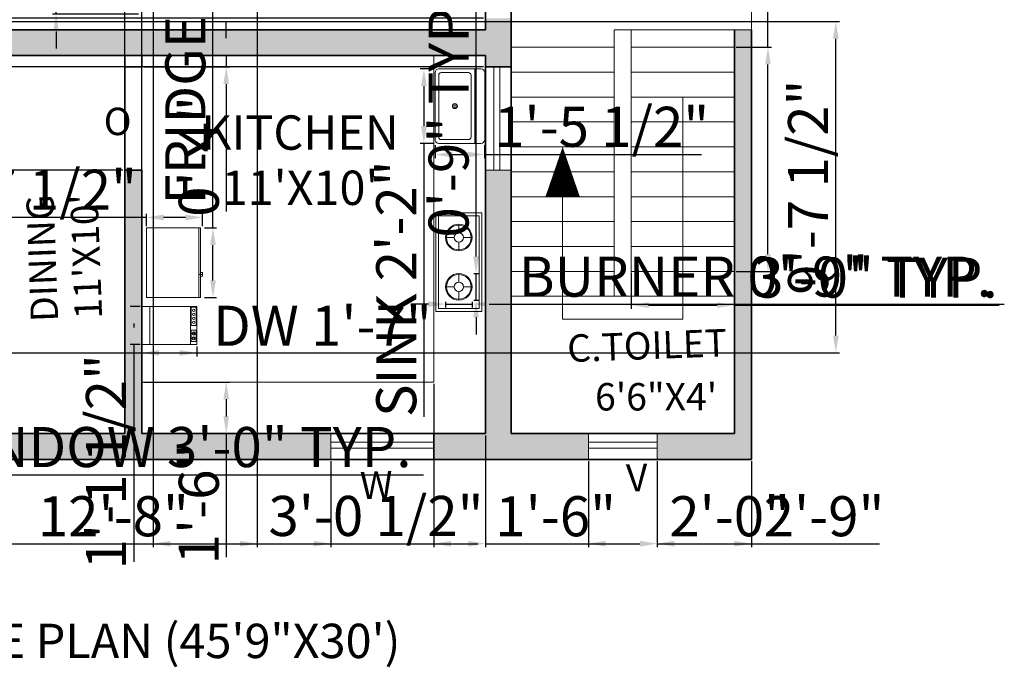
# Model space of a CAD drawing. Units: inches. Extents: x 2961 to 3748, y 1432 to 1961.
# Tile 8 of 9: x 3348 to 3692, y 1432 to 1658. Entities that reach past the tile are written whole.
import ezdxf
from ezdxf.enums import TextEntityAlignment as Align

# ---------------------------------------------------------------- set-up
doc = ezdxf.new("R2010")
doc.units = ezdxf.units.IN
doc.linetypes.add('ACAD_ISO03W100', pattern=[30, 12, -18])
for name, color, linetype, lineweight in [('A-ANNO-DIMS', 2, 'Continuous', 18), ('A-ANNO-TEXT', 7, 'Continuous', 18), ('A-ANNO-TITL', 7, 'Continuous', 25), ('A-AREA-IDEN', 7, 'Continuous', 18), ('A-EQPM', 8, 'Continuous', 18), ('A-FLOR-FIXT', 9, 'Continuous', 18), ('A-FLOR-STRS', 7, 'Continuous', 18), ('A-FURN-FIXD', 9, 'Continuous', 20), ('A-GLAZ', 4, 'Continuous', 18), ('A-ROOF-OVHD', 8, 'ACAD_ISO03W100', 18), ('A-WALL', 7, 'Continuous', 35), ('A-WALL-PATT', 252, 'Continuous', 13)]:
    doc.layers.add(name, color=color, linetype=linetype, lineweight=lineweight)
doc.styles.get("Standard").update_dxf_attribs({"font": 'arial.ttf'})
doc.dimstyles.new('ISO-25', dxfattribs={"dimtxt": 14, "dimasz": 6, "dimexe": 1.25, "dimexo": 0.625, "dimtad": 1, "dimlunit": 3, "dimtxsty": 'Standard', "dimcen": 2.5, "dimadec": 0, "dimazin": 0, "dimtfac": 1, "dimtmove": 0, "dimatfit": 3, "dimfxl": 1, "dimarcsym": 0})

# ---------------------------------------------------------------- blocks, each defined once
blk = doc.blocks.new('Dishwasher')
for p, q in [((16, 32.5), (16.75, 32.5)), ((16.5, 32), (16.2942, 31.7942)), ((16.3156, 33.1843), (16.5, 33)), ((17, 32.75), (17, 33.5)), ((17, 32.25), (17, 31.5)), ((18, 32.5), (17.25, 32.5)), ((17.5, 33), (17.6938, 33.1938)), ((17.7061, 31.7939), (17.5, 32)), ((19, 32.5), (19.75, 32.5)), ((19.5, 32), (19.2942, 31.7942)), ((19.3156, 33.1843), (19.5, 33)), ((20, 32.75), (20, 33.5)), ((20, 32.25), (20, 31.5)), ((21, 32.5), (20.25, 32.5)), ((20.5, 33), (20.6938, 33.1938)), ((20.7061, 31.7939), (20.5, 32)), ((24, 30.5), (0, 30.5)), ((0, 5), (24, 5))]:
    blk.add_line(p, q)
for points in [[(0, 0), (0, 34.5), (24, 34.5), (24, 0)], [(0.5, 31), (0.5, 34), (12, 34), (12, 31)], [(15, 31), (15, 34), (22, 34), (22, 31)]]:
    blk.add_lwpolyline(points, close=True)
for centre, radius in [((2.5, 32.5), 0.75), ((5, 32.5), 0.75), ((7.5, 32.5), 0.75), ((10, 32.5), 0.75), ((17, 32.5), 1), ((20, 32.5), 1)]:
    blk.add_circle(centre, radius)
blk = doc.blocks.new('Refrigerator-2 door - 36 in top')
for p, q in [((0, -26.999999), (36, -26.999999)), ((11, -27.999999), (11, -28.999999)), ((11, -28.999999), (13, -28.999999)), ((12, -26.999999), (12, -28.999999)), ((13, -28.999999), (13, -27.999999))]:
    blk.add_line(p, q)
blk.add_lwpolyline([(0, -27.999999), (0, 0), (36, 0), (36, -27.999999)], close=True)
blk = doc.blocks.new('Sink-single - 30 in top')
blk.add_line((-15, -3.999996), (15, -3.999996))
for points in [[(-13.5, 0), (13.5, 0)], [(-15, -18.499996), (-15, -1.5)], [(15, -1.5), (15, -18.499996)], [(-13.5, -17.499996), (-13.5, -6.499996)], [(-12.5, -5.499996), (12.5, -5.499996)], [(13.5, -6.499996), (13.5, -17.499996)], [(12.5, -18.499996), (-12.5, -18.499996)], [(13.5, -19.999996), (-13.5, -19.999996)]]:
    blk.add_lwpolyline(points)
for radius in [1, 0.5]:
    blk.add_circle((0, -11.999996), radius)
for centre, radius, start, end in [((-13.5, -1.5), 1.5, 90, 180), ((13.5, -1.5), 1.5, 0, 90), ((-12.5, -6.499996), 1, 90, 180), ((12.5, -6.499996), 1, 0, 90), ((-13.5, -18.499996), 1.5, 180, 270), ((-12.5, -17.499996), 1, 180, 270), ((12.5, -17.499996), 1, 270, 0), ((13.5, -18.499996), 1.5, 270, 0)]:
    blk.add_arc(centre, radius, start, end)
blk = doc.blocks.new('WIN-36IN')
for p, q in [((0, 6), (36, 6)), ((0, 3.9), (36, 3.9))]:
    blk.add_line(p, q)
blk.add_lwpolyline([(36, 9), (0, 9), (0, 0), (36, 0)], close=True)
blk = doc.blocks.new('HOB-BURNER')
for p, q in [((4.62, 6.22), (4.62, 9.24)), ((3.02, 4.62), (0, 4.62)), ((9.24, 4.62), (6.22, 4.62)), ((4.62, 0), (4.62, 3.02))]:
    blk.add_line(p, q)
for radius in [4.62, 4.32, 1.6]:
    blk.add_circle((4.62, 4.62), radius)
blk = doc.blocks.new('STAIR-FLIGHT-36IN')
for p, q in [((36, 78.3), (0, 78.3)), ((36, 69.6), (0, 69.6)), ((36, 60.9), (0, 60.9)), ((36, 52.2), (0, 52.2)), ((36, 43.5), (0, 43.5)), ((36, 34.8), (0, 34.8)), ((36, 26.1), (0, 26.1)), ((36, 17.4), (0, 17.4)), ((36, 8.7), (0, 8.7)), ((36, 0), (0, 0)), ((36, 0), (0, 0))]:
    blk.add_line(p, q)
blk = doc.blocks.new('*D20')
at = {"layer": 'A-ANNO-DIMS', "color": 0, "lineweight": -2, "transparency": 16777216}
for p, q in [((3268.27, 1504.01), (3268.27, 1497.99)), ((3304.27, 1504.01), (3304.27, 1497.99)), ((3274.27, 1499.24), (3298.27, 1499.24)), ((3304.27, 1499.24), (3488.68, 1499.24))]:
    blk.add_line(p, q, dxfattribs=at)
at = {"layer": 'A-ANNO-DIMS', "color": 0, "transparency": 16777216}
for points in [[(3274.27, 1500.24), (3274.27, 1498.24), (3268.27, 1499.24)], [(3298.27, 1500.24), (3298.27, 1498.24), (3304.27, 1499.24)]]:
    blk.add_solid(points, dxfattribs=at)
at = {"layer": 'Defpoints', "color": 0, "transparency": 16777216}
for p in [(3268.27, 1504.64), (3304.27, 1504.64), (3304.27, 1499.24)]:
    blk.add_point(p, dxfattribs=at)
at = {"layer": 'A-ANNO-DIMS', "color": 0, "transparency": 16777216, "insert": (3399.47, 1507.11), "char_height": 14, "attachment_point": 5}
blk.add_mtext('WINDOW 3\'-0" TYP.', dxfattribs=at)
blk = doc.blocks.new('*D34')
at = {"layer": 'A-ANNO-DIMS', "color": 0, "lineweight": -2, "transparency": 16777216}
for p, q in [((3490.37, 1558.86), (3484.37, 1558.86)), ((3496.37, 1559.62), (3496.37, 1557.61)), ((3496.37, 1558.86), (3505.61, 1558.86)), ((3505.61, 1559.62), (3505.61, 1557.61)), ((3511.61, 1558.86), (3691.6, 1558.86))]:
    blk.add_line(p, q, dxfattribs=at)
at = {"layer": 'A-ANNO-DIMS', "color": 0, "transparency": 16777216}
for points in [[(3490.37, 1559.86), (3490.37, 1557.86), (3496.37, 1558.86)], [(3511.61, 1559.86), (3511.61, 1557.86), (3505.61, 1558.86)]]:
    blk.add_solid(points, dxfattribs=at)
at = {"layer": 'Defpoints', "color": 0, "transparency": 16777216}
for p in [(3496.37, 1560.25), (3505.61, 1560.25), (3505.61, 1558.86)]:
    blk.add_point(p, dxfattribs=at)
at = {"layer": 'A-ANNO-DIMS', "color": 0, "transparency": 16777216, "insert": (3604.6, 1566.63), "char_height": 14, "attachment_point": 5}
blk.add_mtext('BURNER 0\'-9" TYP.', dxfattribs=at)
blk = doc.blocks.new('*D35')
at = {"layer": 'A-ANNO-DIMS', "color": 0, "lineweight": -2, "transparency": 16777216}
for p, q in [((3507, 1575.49), (3507, 1668.08)), ((3506.23, 1569.49), (3508.25, 1569.49)), ((3507, 1560.25), (3507, 1569.49)), ((3506.23, 1560.25), (3508.25, 1560.25)), ((3507, 1554.25), (3507, 1548.25))]:
    blk.add_line(p, q, dxfattribs=at)
at = {"layer": 'A-ANNO-DIMS', "color": 0, "transparency": 16777216}
for points in [[(3506, 1575.49), (3508, 1575.49), (3507, 1569.49)], [(3506, 1554.25), (3508, 1554.25), (3507, 1560.25)]]:
    blk.add_solid(points, dxfattribs=at)
at = {"layer": 'Defpoints', "color": 0, "transparency": 16777216}
for p in [(3505.61, 1569.49), (3507, 1569.49), (3505.61, 1560.25)]:
    blk.add_point(p, dxfattribs=at)
at = {"layer": 'A-ANNO-DIMS', "color": 0, "transparency": 16777216, "insert": (3499.22, 1624.78), "char_height": 14, "attachment_point": 5, "rotation": 90}
blk.add_mtext('0\'-9" TYP.', dxfattribs=at)
blk = doc.blocks.new('*D36')
at = {"layer": 'A-ANNO-DIMS', "color": 0, "lineweight": -2, "transparency": 16777216}
for p, q in [((3609.01, 1648.54), (3609.01, 1911.68)), ((3597.89, 1648.54), (3610.26, 1648.54)), ((3609.01, 1576.24), (3609.01, 1642.54)), ((3597.89, 1570.24), (3610.26, 1570.24))]:
    blk.add_line(p, q, dxfattribs=at)
at = {"layer": 'A-ANNO-DIMS', "color": 0, "transparency": 16777216}
for points in [[(3608.01, 1642.54), (3610.01, 1642.54), (3609.01, 1648.54)], [(3608.01, 1576.24), (3610.01, 1576.24), (3609.01, 1570.24)]]:
    blk.add_solid(points, dxfattribs=at)
at = {"layer": 'Defpoints', "color": 0, "transparency": 16777216}
for p in [(3597.27, 1648.54), (3609.01, 1648.54), (3597.27, 1570.24)]:
    blk.add_point(p, dxfattribs=at)
at = {"layer": 'A-ANNO-DIMS', "color": 0, "transparency": 16777216, "insert": (3601.15, 1783.11), "char_height": 14, "attachment_point": 5, "rotation": 90}
blk.add_mtext('STAIR FLIGHT 6\'-6 1/2" TYP.', dxfattribs=at)
blk = doc.blocks.new('*D37')
at = {"layer": 'A-ANNO-DIMS', "color": 0, "lineweight": -2, "transparency": 16777216}
for p, q in [((3561.27, 1569.61), (3561.27, 1557.24)), ((3597.27, 1569.61), (3597.27, 1557.24)), ((3567.27, 1558.49), (3591.27, 1558.49)), ((3597.27, 1558.49), (3689.84, 1558.49))]:
    blk.add_line(p, q, dxfattribs=at)
at = {"layer": 'A-ANNO-DIMS', "color": 0, "transparency": 16777216}
for points in [[(3567.27, 1559.49), (3567.27, 1557.49), (3561.27, 1558.49)], [(3591.27, 1559.49), (3591.27, 1557.49), (3597.27, 1558.49)]]:
    blk.add_solid(points, dxfattribs=at)
at = {"layer": 'Defpoints', "color": 0, "transparency": 16777216}
for p in [(3561.27, 1570.24), (3597.27, 1570.24), (3597.27, 1558.49)]:
    blk.add_point(p, dxfattribs=at)
at = {"layer": 'A-ANNO-DIMS', "color": 0, "transparency": 16777216, "insert": (3646.56, 1566.27), "char_height": 14, "attachment_point": 5}
blk.add_mtext('3\'-0" TYP.', dxfattribs=at)
blk = doc.blocks.new('*D38')
at = {"layer": 'A-ANNO-DIMS', "color": 0, "lineweight": -2, "transparency": 16777216}
for p, q in [((3390.27, 1544.05), (3390.27, 1540.55)), ((3396.27, 1541.8), (3403.45, 1541.8)), ((3409.45, 1544.05), (3409.45, 1540.55)), ((3409.45, 1541.8), (3491.24, 1541.8))]:
    blk.add_line(p, q, dxfattribs=at)
at = {"layer": 'A-ANNO-DIMS', "color": 0, "transparency": 16777216}
for points in [[(3396.27, 1542.8), (3396.27, 1540.8), (3390.27, 1541.8)], [(3403.45, 1542.8), (3403.45, 1540.8), (3409.45, 1541.8)]]:
    blk.add_solid(points, dxfattribs=at)
at = {"layer": 'Defpoints', "color": 0, "transparency": 16777216}
for p in [(3390.27, 1544.68), (3409.45, 1544.68), (3409.45, 1541.8)]:
    blk.add_point(p, dxfattribs=at)
at = {"layer": 'A-ANNO-DIMS', "color": 0, "transparency": 16777216, "insert": (3453.35, 1549.46), "char_height": 14, "attachment_point": 5}
blk.add_mtext('DW 1\'-7"', dxfattribs=at)
blk = doc.blocks.new('*D39')
at = {"layer": 'A-ANNO-DIMS', "color": 0, "lineweight": -2, "transparency": 16777216}
for p, q in [((3389.64, 1558.03), (3386.14, 1558.03)), ((3387.39, 1552.03), (3387.39, 1550.68)), ((3389.64, 1544.68), (3386.14, 1544.68)), ((3387.39, 1544.68), (3387.39, 1468.91))]:
    blk.add_line(p, q, dxfattribs=at)
at = {"layer": 'A-ANNO-DIMS', "color": 0, "transparency": 16777216}
for points in [[(3386.39, 1552.03), (3388.39, 1552.03), (3387.39, 1558.03)], [(3386.39, 1550.68), (3388.39, 1550.68), (3387.39, 1544.68)]]:
    blk.add_solid(points, dxfattribs=at)
at = {"layer": 'Defpoints', "color": 0, "transparency": 16777216}
for p in [(3390.27, 1558.03), (3387.39, 1544.68), (3390.27, 1544.68)]:
    blk.add_point(p, dxfattribs=at)
at = {"layer": 'A-ANNO-DIMS', "color": 0, "transparency": 16777216, "insert": (3379.52, 1503.79), "char_height": 14, "attachment_point": 5, "rotation": 90}
blk.add_mtext('1\'-1 1/2"', dxfattribs=at)
blk = doc.blocks.new('*D40')
at = {"layer": 'A-ANNO-DIMS', "color": 0, "lineweight": -2, "transparency": 16777216}
for p, q in [((3415.09, 1585.45), (3415.09, 1741.07)), ((3412.07, 1585.45), (3416.34, 1585.45)), ((3415.09, 1567.11), (3415.09, 1579.45)), ((3412.07, 1561.11), (3416.34, 1561.11))]:
    blk.add_line(p, q, dxfattribs=at)
at = {"layer": 'A-ANNO-DIMS', "color": 0, "transparency": 16777216}
for points in [[(3414.09, 1579.45), (3416.09, 1579.45), (3415.09, 1585.45)], [(3414.09, 1567.11), (3416.09, 1567.11), (3415.09, 1561.11)]]:
    blk.add_solid(points, dxfattribs=at)
at = {"layer": 'Defpoints', "color": 0, "transparency": 16777216}
for p in [(3411.44, 1585.45), (3415.09, 1585.45), (3411.44, 1561.11)]:
    blk.add_point(p, dxfattribs=at)
at = {"layer": 'A-ANNO-DIMS', "color": 0, "transparency": 16777216, "insert": (3407.23, 1666.26), "char_height": 14, "attachment_point": 5, "rotation": 90}
blk.add_mtext('FRIDGE 2\'-0 1/2"', dxfattribs=at)
blk = doc.blocks.new('*D41')
at = {"layer": 'A-ANNO-DIMS', "color": 0, "lineweight": -2, "transparency": 16777216}
for p, q in [((3391.84, 1586.08), (3391.84, 1590.35)), ((3411.44, 1586.08), (3411.44, 1590.35)), ((3391.84, 1589.1), (3316.07, 1589.1)), ((3405.44, 1589.1), (3397.84, 1589.1))]:
    blk.add_line(p, q, dxfattribs=at)
at = {"layer": 'A-ANNO-DIMS', "color": 0, "transparency": 16777216}
for points in [[(3397.84, 1590.1), (3397.84, 1588.1), (3391.84, 1589.1)], [(3405.44, 1590.1), (3405.44, 1588.1), (3411.44, 1589.1)]]:
    blk.add_solid(points, dxfattribs=at)
at = {"layer": 'Defpoints', "color": 0, "transparency": 16777216}
for p in [(3391.84, 1589.1), (3391.84, 1585.45), (3411.44, 1585.45)]:
    blk.add_point(p, dxfattribs=at)
at = {"layer": 'A-ANNO-DIMS', "color": 0, "transparency": 16777216, "insert": (3350.95, 1596.96), "char_height": 14, "attachment_point": 5}
blk.add_mtext('1\'-7 1/2"', dxfattribs=at)
blk = doc.blocks.new('*D42')
at = {"layer": 'A-ANNO-DIMS', "color": 0, "lineweight": -2, "transparency": 16777216}
for p, q in [((3492.07, 1640.96), (3487.54, 1640.96)), ((3488.79, 1634.96), (3488.79, 1620.96)), ((3492.07, 1614.96), (3487.54, 1614.96)), ((3488.79, 1614.96), (3488.79, 1519.48))]:
    blk.add_line(p, q, dxfattribs=at)
at = {"layer": 'A-ANNO-DIMS', "color": 0, "transparency": 16777216}
for points in [[(3487.79, 1634.96), (3489.79, 1634.96), (3488.79, 1640.96)], [(3487.79, 1620.96), (3489.79, 1620.96), (3488.79, 1614.96)]]:
    blk.add_solid(points, dxfattribs=at)
at = {"layer": 'Defpoints', "color": 0, "transparency": 16777216}
for p in [(3492.69, 1640.96), (3488.79, 1614.96), (3492.69, 1614.96)]:
    blk.add_point(p, dxfattribs=at)
at = {"layer": 'A-ANNO-DIMS', "color": 0, "transparency": 16777216, "insert": (3480.93, 1564.22), "char_height": 14, "attachment_point": 5, "rotation": 90}
blk.add_mtext('SINK 2\'-2"', dxfattribs=at)
blk = doc.blocks.new('*D43')
at = {"layer": 'A-ANNO-DIMS', "color": 0, "lineweight": -2, "transparency": 16777216}
for p, q in [((3492.69, 1614.34), (3492.69, 1609.81)), ((3510.02, 1614.34), (3510.02, 1609.81)), ((3498.69, 1611.06), (3504.02, 1611.06)), ((3510.02, 1611.06), (3585.79, 1611.06))]:
    blk.add_line(p, q, dxfattribs=at)
at = {"layer": 'A-ANNO-DIMS', "color": 0, "transparency": 16777216}
for points in [[(3498.69, 1612.06), (3498.69, 1610.06), (3492.69, 1611.06)], [(3504.02, 1612.06), (3504.02, 1610.06), (3510.02, 1611.06)]]:
    blk.add_solid(points, dxfattribs=at)
at = {"layer": 'Defpoints', "color": 0, "transparency": 16777216}
for p in [(3492.69, 1614.96), (3510.02, 1614.96), (3510.02, 1611.06)]:
    blk.add_point(p, dxfattribs=at)
at = {"layer": 'A-ANNO-DIMS', "color": 0, "transparency": 16777216, "insert": (3550.91, 1618.93), "char_height": 14, "attachment_point": 5}
blk.add_mtext('1\'-5 1/2"', dxfattribs=at)
blk = doc.blocks.new('*D51')
at = {"layer": 'A-ANNO-DIMS', "color": 0, "lineweight": -2, "transparency": 16777216}
for p, q in [((3390.89, 1531.64), (3420.97, 1531.64)), ((3419.72, 1525.64), (3419.72, 1519.64)), ((3390.89, 1513.64), (3420.97, 1513.64)), ((3419.72, 1513.64), (3419.72, 1470.49))]:
    blk.add_line(p, q, dxfattribs=at)
at = {"layer": 'A-ANNO-DIMS', "color": 0, "transparency": 16777216}
for points in [[(3418.72, 1525.64), (3420.72, 1525.64), (3419.72, 1531.64)], [(3418.72, 1519.64), (3420.72, 1519.64), (3419.72, 1513.64)]]:
    blk.add_solid(points, dxfattribs=at)
at = {"layer": 'Defpoints', "color": 0, "transparency": 16777216}
for p in [(3390.27, 1531.64), (3390.27, 1513.64), (3419.72, 1513.64)]:
    blk.add_point(p, dxfattribs=at)
at = {"layer": 'A-ANNO-DIMS', "color": 0, "transparency": 16777216, "insert": (3411.94, 1489.06), "char_height": 14, "attachment_point": 5, "rotation": 90}
blk.add_mtext('1\'-6"', dxfattribs=at)
blk = doc.blocks.new('*D52')
at = {"layer": 'A-ANNO-DIMS', "color": 0, "lineweight": -2, "transparency": 16777216}
for p, q in [((3360.27, 1678.21), (3360.27, 1721.36)), ((3389.1, 1672.21), (3359.02, 1672.21)), ((3360.27, 1660.05), (3360.27, 1672.21)), ((3389.1, 1660.05), (3359.02, 1660.05)), ((3360.27, 1654.05), (3360.27, 1648.05))]:
    blk.add_line(p, q, dxfattribs=at)
at = {"layer": 'A-ANNO-DIMS', "color": 0, "transparency": 16777216}
for points in [[(3359.27, 1678.21), (3361.27, 1678.21), (3360.27, 1672.21)], [(3359.27, 1654.05), (3361.27, 1654.05), (3360.27, 1660.05)]]:
    blk.add_solid(points, dxfattribs=at)
at = {"layer": 'Defpoints', "color": 0, "transparency": 16777216}
for p in [(3360.27, 1672.21), (3389.72, 1672.21), (3389.72, 1660.05)]:
    blk.add_point(p, dxfattribs=at)
at = {"layer": 'A-ANNO-DIMS', "color": 0, "transparency": 16777216, "insert": (3352.5, 1702.78), "char_height": 14, "attachment_point": 5, "rotation": 90}
blk.add_mtext('1\'-0"', dxfattribs=at)
blk = doc.blocks.new('*D58')
at = {"layer": 'A-ANNO-DIMS', "color": 0, "lineweight": -2, "transparency": 16777216}
for p, q in [((3304.27, 1504.01), (3304.27, 1473.94)), ((3456.27, 1504.01), (3456.27, 1473.94)), ((3310.27, 1475.19), (3450.27, 1475.19))]:
    blk.add_line(p, q, dxfattribs=at)
at = {"layer": 'A-ANNO-DIMS', "color": 0, "transparency": 16777216}
for points in [[(3310.27, 1476.19), (3310.27, 1474.19), (3304.27, 1475.19)], [(3450.27, 1476.19), (3450.27, 1474.19), (3456.27, 1475.19)]]:
    blk.add_solid(points, dxfattribs=at)
at = {"layer": 'Defpoints', "color": 0, "transparency": 16777216}
for p in [(3304.27, 1504.64), (3456.27, 1504.64), (3456.27, 1475.19)]:
    blk.add_point(p, dxfattribs=at)
at = {"layer": 'A-ANNO-DIMS', "color": 0, "transparency": 16777216, "insert": (3380.27, 1482.96), "char_height": 14, "attachment_point": 5}
blk.add_mtext('12\'-8"', dxfattribs=at)
blk = doc.blocks.new('*D59')
at = {"layer": 'A-ANNO-DIMS', "color": 0, "lineweight": -2, "transparency": 16777216}
for p, q in [((3570.27, 1504.01), (3570.27, 1473.94)), ((3603.27, 1504.01), (3603.27, 1473.94)), ((3576.27, 1475.19), (3597.27, 1475.19)), ((3603.27, 1475.19), (3647.97, 1475.19))]:
    blk.add_line(p, q, dxfattribs=at)
at = {"layer": 'A-ANNO-DIMS', "color": 0, "transparency": 16777216}
for points in [[(3576.27, 1476.19), (3576.27, 1474.19), (3570.27, 1475.19)], [(3597.27, 1476.19), (3597.27, 1474.19), (3603.27, 1475.19)]]:
    blk.add_solid(points, dxfattribs=at)
at = {"layer": 'Defpoints', "color": 0, "transparency": 16777216}
for p in [(3570.27, 1504.64), (3603.27, 1504.64), (3603.27, 1475.19)]:
    blk.add_point(p, dxfattribs=at)
at = {"layer": 'A-ANNO-DIMS', "color": 0, "transparency": 16777216, "insert": (3628.62, 1482.96), "char_height": 14, "attachment_point": 5}
blk.add_mtext('2\'-9"', dxfattribs=at)
blk = doc.blocks.new('*D60')
at = {"layer": 'A-ANNO-DIMS', "color": 0, "lineweight": -2, "transparency": 16777216}
for p, q in [((3546.27, 1504.01), (3546.27, 1473.94)), ((3570.27, 1504.01), (3570.27, 1473.94)), ((3552.27, 1475.19), (3564.27, 1475.19)), ((3570.27, 1475.19), (3614.97, 1475.19))]:
    blk.add_line(p, q, dxfattribs=at)
at = {"layer": 'A-ANNO-DIMS', "color": 0, "transparency": 16777216}
for points in [[(3552.27, 1476.19), (3552.27, 1474.19), (3546.27, 1475.19)], [(3564.27, 1476.19), (3564.27, 1474.19), (3570.27, 1475.19)]]:
    blk.add_solid(points, dxfattribs=at)
at = {"layer": 'Defpoints', "color": 0, "transparency": 16777216}
for p in [(3546.27, 1504.64), (3570.27, 1504.64), (3570.27, 1475.19)]:
    blk.add_point(p, dxfattribs=at)
at = {"layer": 'A-ANNO-DIMS', "color": 0, "transparency": 16777216, "insert": (3595.62, 1482.96), "char_height": 14, "attachment_point": 5}
blk.add_mtext('2\'-0"', dxfattribs=at)
blk = doc.blocks.new('*D68')
at = {"layer": 'A-ANNO-DIMS', "color": 0, "lineweight": -2, "transparency": 16777216}
for p, q in [((3024.82, 1658.64), (3024.82, 1701.79)), ((3509.64, 1658.64), (3023.57, 1658.64)), ((3024.82, 1647.64), (3024.82, 1652.64)), ((3509.64, 1641.64), (3023.57, 1641.64))]:
    blk.add_line(p, q, dxfattribs=at)
at = {"layer": 'A-ANNO-DIMS', "color": 0, "transparency": 16777216}
for points in [[(3023.82, 1652.64), (3025.82, 1652.64), (3024.82, 1658.64)], [(3023.82, 1647.64), (3025.82, 1647.64), (3024.82, 1641.64)]]:
    blk.add_solid(points, dxfattribs=at)
at = {"layer": 'Defpoints', "color": 0, "transparency": 16777216}
for p in [(3024.82, 1658.64), (3510.27, 1658.64), (3510.27, 1641.64)]:
    blk.add_point(p, dxfattribs=at)
at = {"layer": 'A-ANNO-DIMS', "color": 0, "transparency": 16777216, "insert": (3017.04, 1683.21), "char_height": 14, "attachment_point": 5, "rotation": 90}
blk.add_mtext('1\'-5"', dxfattribs=at)
blk = doc.blocks.new('*D70')
at = {"layer": 'A-ANNO-DIMS', "color": 0, "lineweight": -2, "transparency": 16777216}
for p, q in [((3024.82, 1641.64), (3024.82, 1686.09)), ((3383.64, 1641.64), (3023.57, 1641.64)), ((3024.82, 1611.64), (3024.82, 1635.64)), ((3383.64, 1605.64), (3023.57, 1605.64))]:
    blk.add_line(p, q, dxfattribs=at)
at = {"layer": 'A-ANNO-DIMS', "color": 0, "transparency": 16777216}
for points in [[(3023.82, 1635.64), (3025.82, 1635.64), (3024.82, 1641.64)], [(3023.82, 1611.64), (3025.82, 1611.64), (3024.82, 1605.64)]]:
    blk.add_solid(points, dxfattribs=at)
at = {"layer": 'Defpoints', "color": 0, "transparency": 16777216}
for p in [(3024.82, 1641.64), (3384.27, 1641.64), (3384.27, 1605.64)]:
    blk.add_point(p, dxfattribs=at)
at = {"layer": 'A-ANNO-DIMS', "color": 0, "transparency": 16777216, "insert": (3017.04, 1666.87), "char_height": 14, "attachment_point": 5, "rotation": 90}
blk.add_mtext('3\'-0"', dxfattribs=at)
blk = doc.blocks.new('*D78')
at = {"layer": 'A-ANNO-DIMS', "color": 0, "lineweight": -2, "transparency": 16777216}
for p, q in [((3394.23, 1792.44), (3394.23, 1473.94)), ((3430.5, 1792.44), (3430.5, 1473.94)), ((3400.23, 1475.19), (3424.5, 1475.19)), ((3430.5, 1475.19), (3507.58, 1475.19))]:
    blk.add_line(p, q, dxfattribs=at)
at = {"layer": 'A-ANNO-DIMS', "color": 0, "transparency": 16777216}
for points in [[(3400.23, 1476.19), (3400.23, 1474.19), (3394.23, 1475.19)], [(3424.5, 1476.19), (3424.5, 1474.19), (3430.5, 1475.19)]]:
    blk.add_solid(points, dxfattribs=at)
at = {"layer": 'Defpoints', "color": 0, "transparency": 16777216}
for p in [(3394.23, 1793.06), (3430.5, 1793.06), (3430.5, 1475.19)]:
    blk.add_point(p, dxfattribs=at)
at = {"layer": 'A-ANNO-DIMS', "color": 0, "transparency": 16777216, "insert": (3472.04, 1483.06), "char_height": 14, "attachment_point": 5}
blk.add_mtext('3\'-0 1/2"', dxfattribs=at)
blk = doc.blocks.new('*D81')
at = {"layer": 'A-ANNO-DIMS', "color": 0, "lineweight": -2, "transparency": 16777216}
for p, q in [((3063.89, 1657.48), (3633.97, 1657.48)), ((3632.72, 1547.87), (3632.72, 1651.48)), ((3063.89, 1541.87), (3633.97, 1541.87))]:
    blk.add_line(p, q, dxfattribs=at)
at = {"layer": 'A-ANNO-DIMS', "color": 0, "transparency": 16777216}
for points in [[(3631.72, 1651.48), (3633.72, 1651.48), (3632.72, 1657.48)], [(3631.72, 1547.87), (3633.72, 1547.87), (3632.72, 1541.87)]]:
    blk.add_solid(points, dxfattribs=at)
at = {"layer": 'Defpoints', "color": 0, "transparency": 16777216}
for p in [(3063.27, 1657.48), (3632.72, 1657.48), (3063.27, 1541.87)]:
    blk.add_point(p, dxfattribs=at)
at = {"layer": 'A-ANNO-DIMS', "color": 0, "transparency": 16777216, "insert": (3624.85, 1599.67), "char_height": 14, "attachment_point": 5, "rotation": 90}
blk.add_mtext('9\'-7 1/2"', dxfattribs=at)
blk = doc.blocks.new('*D87')
at = {"layer": 'A-ANNO-DIMS', "color": 0, "lineweight": -2, "transparency": 16777216}
for p, q in [((3384.27, 1514.26), (3384.27, 1933.63)), ((3390.27, 1514.26), (3390.27, 1933.63)), ((3378.27, 1932.38), (3372.27, 1932.38)), ((3384.27, 1932.38), (3390.27, 1932.38)), ((3396.27, 1932.38), (3440.73, 1932.38))]:
    blk.add_line(p, q, dxfattribs=at)
at = {"layer": 'A-ANNO-DIMS', "color": 0, "transparency": 16777216}
for points in [[(3378.27, 1933.38), (3378.27, 1931.38), (3384.27, 1932.38)], [(3396.27, 1933.38), (3396.27, 1931.38), (3390.27, 1932.38)]]:
    blk.add_solid(points, dxfattribs=at)
at = {"layer": 'Defpoints', "color": 0, "transparency": 16777216}
for p in [(3390.27, 1932.38), (3384.27, 1513.64), (3390.27, 1513.64)]:
    blk.add_point(p, dxfattribs=at)
at = {"layer": 'A-ANNO-DIMS', "color": 0, "transparency": 16777216, "insert": (3421.5, 1940.15), "char_height": 14, "attachment_point": 5}
blk.add_mtext('0\'-6"', dxfattribs=at)
blk = doc.blocks.new('*D88')
at = {"layer": 'A-ANNO-DIMS', "color": 0, "lineweight": -2, "transparency": 16777216}
for p, q in [((3492.27, 1531.01), (3492.27, 1473.94)), ((3510.27, 1513.01), (3510.27, 1473.94)), ((3498.27, 1475.19), (3504.27, 1475.19)), ((3510.27, 1475.19), (3553.41, 1475.19))]:
    blk.add_line(p, q, dxfattribs=at)
at = {"layer": 'A-ANNO-DIMS', "color": 0, "transparency": 16777216}
for points in [[(3498.27, 1476.19), (3498.27, 1474.19), (3492.27, 1475.19)], [(3504.27, 1476.19), (3504.27, 1474.19), (3510.27, 1475.19)]]:
    blk.add_solid(points, dxfattribs=at)
at = {"layer": 'Defpoints', "color": 0, "transparency": 16777216}
for p in [(3492.27, 1531.64), (3510.27, 1513.64), (3510.27, 1475.19)]:
    blk.add_point(p, dxfattribs=at)
at = {"layer": 'A-ANNO-DIMS', "color": 0, "transparency": 16777216, "insert": (3534.84, 1482.96), "char_height": 14, "attachment_point": 5}
blk.add_mtext('1\'-6"', dxfattribs=at)
blk = doc.blocks.new('*D90')
at = {"layer": 'A-ANNO-DIMS', "color": 0, "lineweight": -2, "transparency": 16777216}
for p, q in [((3419.72, 1651.64), (3419.72, 1657.64)), ((3390.89, 1645.64), (3420.97, 1645.64)), ((3419.72, 1645.64), (3419.72, 1641.64)), ((3390.89, 1641.64), (3420.97, 1641.64)), ((3419.72, 1635.64), (3419.72, 1591.17))]:
    blk.add_line(p, q, dxfattribs=at)
at = {"layer": 'A-ANNO-DIMS', "color": 0, "transparency": 16777216}
for points in [[(3418.72, 1651.64), (3420.72, 1651.64), (3419.72, 1645.64)], [(3418.72, 1635.64), (3420.72, 1635.64), (3419.72, 1641.64)]]:
    blk.add_solid(points, dxfattribs=at)
at = {"layer": 'Defpoints', "color": 0, "transparency": 16777216}
for p in [(3390.27, 1645.64), (3390.27, 1641.64), (3419.72, 1641.64)]:
    blk.add_point(p, dxfattribs=at)
at = {"layer": 'A-ANNO-DIMS', "color": 0, "transparency": 16777216, "insert": (3411.94, 1610.41), "char_height": 14, "attachment_point": 5, "rotation": 90}
blk.add_mtext('0\'-4"', dxfattribs=at)

msp = doc.modelspace()

# ---------------------------------------------------------------- hatches: boundary and pattern name
at = {"layer": 'A-WALL-PATT'}
h = msp.add_hatch(color=256, dxfattribs=at)
h.set_gradient(color1=(41, 49, 137), color2=(41, 49, 137), tint=1)
h.paths.add_polyline_path([(3255.267, 1671.639), (3255.267, 1513.639), (3251.267, 1513.639), (3251.267, 1504.639), (3268.267, 1504.639), (3268.267, 1513.639), (3264.267, 1513.639), (3264.267, 1671.639), (3259.767, 1671.639)])
h.paths.add_polyline_path([(3063.267, 1513.639), (3063.267, 1677.639), (3054.267, 1677.639), (3054.267, 1504.639), (3215.267, 1504.639), (3215.267, 1513.639)])
h.paths.add_polyline_path([(3304.267, 1513.639), (3304.267, 1504.639), (3456.267, 1504.639), (3456.267, 1513.639), (3390.267, 1513.639), (3390.267, 1605.639), (3384.267, 1605.639), (3384.267, 1513.639)])
h.paths.add_polyline_path([(3510.267, 1605.639), (3510.267, 1513.639), (3492.267, 1513.639), (3492.267, 1504.639), (3546.267, 1504.639), (3546.267, 1513.639), (3519.267, 1513.639), (3519.267, 1605.639)])
h.paths.add_polyline_path([(3340.267, 1654.639), (3340.267, 1645.639), (3510.267, 1645.639), (3510.267, 1641.639), (3519.267, 1641.639), (3519.267, 1658.639), (3510.267, 1658.639), (3510.267, 1654.639)])
h.paths.add_polyline_path([(3223.801, 1864.639), (3223.801, 1855.639), (3255.267, 1855.639), (3255.267, 1772.534), (3264.267, 1772.534), (3264.267, 1855.639), (3303.267, 1855.639), (3303.267, 1864.639)])
h.paths.add_polyline_path([(3339.267, 1864.639), (3339.267, 1855.639), (3435.267, 1855.639), (3435.267, 1864.639)])
h.paths.add_polyline_path([(3471.267, 1864.639), (3471.267, 1855.639), (3510.267, 1855.639), (3510.267, 1827.639), (3519.267, 1827.639), (3519.267, 1864.639)])
h.paths.add_polyline_path([(3510.267, 1767.639), (3510.267, 1739.639), (3519.267, 1739.639), (3519.267, 1767.639)])
h.paths.add_polyline_path([(3123.267, 1726.639), (3123.267, 1855.639), (3187.801, 1855.639), (3187.801, 1864.639), (3054.267, 1864.639), (3054.267, 1837.201), (3063.267, 1837.201), (3063.267, 1855.639), (3117.267, 1855.639), (3117.267, 1726.639), (3103.267, 1726.639), (3103.267, 1717.639), (3255.267, 1717.639), (3255.267, 1713.639), (3264.267, 1713.639), (3264.267, 1730.534), (3255.267, 1730.639), (3255.267, 1726.639)])
h.paths.add_polyline_path([(3597.267, 1654.639), (3597.267, 1513.639), (3570.267, 1513.639), (3570.267, 1504.639), (3603.267, 1504.639), (3603.267, 1654.639)])
h.paths.add_polyline_path([(3054.267, 1813.201), (3054.267, 1713.639), (3063.267, 1713.639), (3063.267, 1717.639), (3069.267, 1717.639), (3069.267, 1726.639), (3063.267, 1726.639), (3063.267, 1813.201)], flags=17)

# ---------------------------------------------------------------- linework, layer by layer
at = {"layer": 'A-EQPM'}
for points in [[(3492.912, 1556.259), (3492.912, 1590.698), (3509.063, 1590.698), (3509.063, 1556.259)], [(3493.912, 1557.259), (3493.912, 1589.698), (3508.063, 1589.698), (3508.063, 1557.259)]]:
    msp.add_lwpolyline(points, close=True, dxfattribs=at)
at = {"layer": 'A-FLOR-STRS'}
for p, q in [((3603.267, 1654.639), (3555.267, 1654.639)), ((3555.267, 1561.639), (3555.267, 1654.639)), ((3561.267, 1561.639), (3561.267, 1654.639)), ((3579.267, 1631.139), (3579.267, 1561.639)), ((3537.267, 1553.526), (3537.267, 1596.339)), ((3597.267, 1561.639), (3519.267, 1561.639)), ((3579.267, 1561.639), (3579.267, 1553.526)), ((3579.267, 1553.526), (3537.267, 1553.526))]:
    msp.add_line(p, q, dxfattribs=at)
msp.add_lwpolyline([(3537.267, 1596.339, 12, 0, 0), (3537.267, 1613.739, 0, 0, 0)], format="xyseb", dxfattribs=at)
at = {"layer": 'A-FURN-FIXD'}
for p in [(3492.267, 1645.639), (3390.267, 1531.639)]:
    msp.add_line(p, (3492.267, 1531.639), dxfattribs=at)
at = {"layer": 'A-GLAZ'}
for p, q in [((3546.267, 1510.639), (3570.267, 1510.639)), ((3546.267, 1508.539), (3570.267, 1508.539))]:
    msp.add_line(p, q, dxfattribs=at)
msp.add_lwpolyline([(3546.267, 1513.639), (3546.267, 1504.639), (3570.267, 1504.639), (3570.267, 1513.639)], close=True, dxfattribs=at)
at = {"layer": 'A-ROOF-OVHD'}
msp.add_line((3603.267, 1654.639), (3603.267, 1864.639), dxfattribs=at)
at = {"layer": 'A-WALL'}
for p, q in [((3519.267, 1513.639), (3519.267, 1864.639)), ((3510.267, 1654.639), (3510.267, 1767.639)), ((3510.267, 1654.639), (3264.267, 1654.639)), ((3597.267, 1513.639), (3597.267, 1654.639)), ((3603.267, 1504.639), (3603.267, 1654.639)), ((3510.267, 1645.639), (3340.267, 1645.639)), ((3384.267, 1513.639), (3384.267, 1645.639)), ((3390.267, 1641.639), (3390.267, 1645.639)), ((3510.267, 1513.639), (3510.267, 1645.639)), ((3390.267, 1641.639), (3384.267, 1641.639)), ((3510.267, 1641.639), (3519.267, 1641.639)), ((3390.267, 1605.639), (3384.267, 1605.639)), ((3390.267, 1513.639), (3390.267, 1605.639)), ((3384.267, 1513.639), (3264.267, 1513.639)), ((3510.267, 1513.639), (3390.267, 1513.639)), ((3492.267, 1513.639), (3492.267, 1504.639)), ((3597.267, 1513.639), (3519.267, 1513.639)), ((3603.267, 1504.639), (3054.267, 1504.639))]:
    msp.add_line(p, q, dxfattribs=at)

# ---------------------------------------------------------------- block references
at = {"layer": 'A-EQPM'}
for p in [(3496.366, 1577.467), (3496.366, 1560.247)]:
    msp.add_blockref('HOB-BURNER', p, dxfattribs=at)
for name, p, xscale, yscale, zscale, rotation in [('Refrigerator-2 door - 36 in top', (3391.836, 1561.114), 0.6760214134564775, 0.6760214134564775, 0.6760214134564775, 90), ('Dishwasher', (3390.267, 1558.025), 0.5561496414596057, 0.5561496414596057, 0.5561496414596057, 269.9999999999999)]:
    msp.add_blockref(name, p, dxfattribs=dict(at, xscale=xscale, yscale=yscale, zscale=zscale, rotation=rotation))
at = {"layer": 'A-FLOR-FIXT', "xscale": 0.8666664000000007, "yscale": 0.8666664000000007, "zscale": 0.8666664000000007, "rotation": 269.9999999999999}
msp.add_blockref('Sink-single - 30 in top', (3510.025, 1627.962), dxfattribs=at)
at = {"layer": 'A-FLOR-STRS'}
for p in [(3519.267, 1570.239), (3561.267, 1570.239)]:
    msp.add_blockref('STAIR-FLIGHT-36IN', p, dxfattribs=at)
at = {"layer": 'A-GLAZ', "rotation": 90.00000000000213}
msp.add_blockref('WIN-36IN', (3519.267, 1605.639), dxfattribs=at)
at = {"layer": 'A-GLAZ'}
msp.add_blockref('WIN-36IN', (3456.267, 1504.639), dxfattribs=at)

# ---------------------------------------------------------------- texts
at = {"layer": 'A-ANNO-TEXT'}
msp.add_text('O', height=9.571, dxfattribs=at).set_placement((3376.938, 1617.838))
for s, p in [('W', (3472.402, 1490.858)), ('V', (3563.423, 1493.454))]:
    msp.add_text(s, height=9.571, rotation=2.15165, dxfattribs=at).set_placement(p, align=Align.CENTER)
at = {"layer": 'A-ANNO-TITL'}
msp.add_text('EAST FACING HOUSE PLAN (45\'9"X30\')', height=12, dxfattribs=at).set_placement((3335.479, 1435.239), align=Align.CENTER)
at = {"layer": 'A-AREA-IDEN'}
for s, p in [('KITCHEN', (3445.515, 1612.731)), ("11'X10'", (3445.515, 1593.454))]:
    msp.add_text(s, height=12, dxfattribs=at).set_placement(p, align=Align.CENTER)
for s, rotation, p in [('DINING', 92.15165, (3360.196, 1575.032)), ("11'X10'", 92.15165, (3375.559, 1575.609)), ('C.TOILET', 2.15165, (3566.972, 1539.606))]:
    msp.add_text(s, height=9.5707, rotation=rotation, dxfattribs=at).set_placement(p, align=Align.CENTER)
msp.add_text('6\'6"X4\'', height=9.5707, dxfattribs=at).set_placement((3548.59, 1521.697))

# ---------------------------------------------------------------- dimensions: what is measured, and where the dimension line sits
at = {"layer": 'A-ANNO-DIMS'}
for base, p1, p2, picture, middle in [((3390.267, 1932.38), (3384.267, 1513.639), (3390.267, 1513.639), '*D87', (3421.5, 1940.153)), ((3430.505, 1475.189), (3394.234, 1793.062), (3430.505, 1793.062), '*D78', (3472.044, 1483.057)), ((3510.025, 1611.062), (3492.691, 1614.962), (3510.025, 1614.962), '*D43', (3550.909, 1618.926)), ((3510.267, 1475.189), (3492.267, 1531.639), (3510.267, 1513.639), '*D88', (3534.841, 1482.962)), ((3456.267, 1475.189), (3304.267, 1504.639), (3456.267, 1504.639), '*D58', (3380.267, 1482.962)), ((3570.267, 1475.189), (3546.267, 1504.639), (3570.267, 1504.639), '*D60', (3595.619, 1482.962)), ((3603.267, 1475.189), (3570.267, 1504.639), (3603.267, 1504.639), '*D59', (3628.619, 1482.962))]:
    dim = msp.add_linear_dim(base=base, p1=p1, p2=p2, dimstyle='ISO-25', override={"dimdec": 1, "dimlfac": 1, "dimrnd": 0, "dimzin": 1, "dimdsep": 46, "dimlunit": 4, "dimfrac": 2}, dxfattribs=at)
    dim.commit()
    dim.dimension.update_dxf_attribs({"geometry": picture, "text_midpoint": middle})
for base, p1, p2, angle, text, picture, middle in [((3609.012, 1648.539), (3597.267, 1570.239), (3597.267, 1648.539), 90, 'STAIR FLIGHT <> TYP.', '*D36', (3601.148, 1783.112)), ((3415.091, 1585.45), (3411.44, 1561.114), (3411.44, 1585.45), 90, 'FRIDGE <>', '*D40', (3407.227, 1666.258)), ((3506.995, 1569.49), (3505.609, 1560.247), (3505.609, 1569.49), 90, '<> TYP.', '*D35', (3499.222, 1624.783)), ((3488.791, 1614.962), (3492.691, 1640.962), (3492.691, 1614.962), 270, 'SINK <>', '*D42', (3480.928, 1564.222))]:
    dim = msp.add_linear_dim(base=base, p1=p1, p2=p2, angle=angle, text=text, dimstyle='ISO-25', override={"dimdec": 1, "dimlfac": 1, "dimrnd": 0, "dimzin": 1, "dimdsep": 46, "dimlunit": 4, "dimfrac": 2}, dxfattribs=at)
    dim.commit()
    dim.dimension.update_dxf_attribs({"geometry": picture, "text_midpoint": middle})
for base, p1, p2, angle, picture, middle in [((3360.274, 1672.208), (3389.724, 1660.049), (3389.724, 1672.208), 90, '*D52', (3352.501, 1702.782)), ((3024.817, 1658.639), (3510.267, 1641.639), (3510.267, 1658.639), 90, '*D68', (3017.044, 1683.212)), ((3024.817, 1641.639), (3384.267, 1605.639), (3384.267, 1641.639), 90, '*D70', (3017.039, 1666.867)), ((3632.717, 1657.476), (3063.267, 1541.867), (3063.267, 1657.476), 90, '*D81', (3624.853, 1599.671)), ((3419.717, 1641.639), (3390.267, 1645.639), (3390.267, 1641.639), 270, '*D90', (3411.944, 1610.406)), ((3391.836, 1589.101), (3411.44, 1585.45), (3391.836, 1585.45), 180, '*D41', (3350.951, 1596.965)), ((3387.389, 1544.677), (3390.267, 1558.025), (3390.267, 1544.677), 270, '*D39', (3379.525, 1503.793)), ((3419.717, 1513.639), (3390.267, 1531.639), (3390.267, 1513.639), 270, '*D51', (3411.944, 1489.065))]:
    dim = msp.add_linear_dim(base=base, p1=p1, p2=p2, angle=angle, dimstyle='ISO-25', override={"dimdec": 1, "dimlfac": 1, "dimrnd": 0, "dimzin": 1, "dimdsep": 46, "dimlunit": 4, "dimfrac": 2}, dxfattribs=at)
    dim.commit()
    dim.dimension.update_dxf_attribs({"geometry": picture, "text_midpoint": middle})
for base, p1, p2, text, picture, middle in [((3505.609, 1558.861), (3496.366, 1560.247), (3505.609, 1560.247), 'BURNER <> TYP.', '*D34', (3604.602, 1566.634)), ((3597.267, 1558.494), (3561.267, 1570.239), (3597.267, 1570.239), '<> TYP.', '*D37', (3646.556, 1566.271)), ((3409.454, 1541.799), (3390.267, 1544.677), (3409.454, 1544.677), 'DW <>', '*D38', (3453.347, 1549.458)), ((3304.267, 1499.239), (3268.267, 1504.639), (3304.267, 1504.639), 'WINDOW <> TYP.', '*D20', (3399.471, 1507.112))]:
    dim = msp.add_linear_dim(base=base, p1=p1, p2=p2, text=text, dimstyle='ISO-25', override={"dimdec": 1, "dimlfac": 1, "dimrnd": 0, "dimzin": 1, "dimdsep": 46, "dimlunit": 4, "dimfrac": 2}, dxfattribs=at)
    dim.commit()
    dim.dimension.update_dxf_attribs({"geometry": picture, "text_midpoint": middle})

doc.saveas('drawing.dxf')
